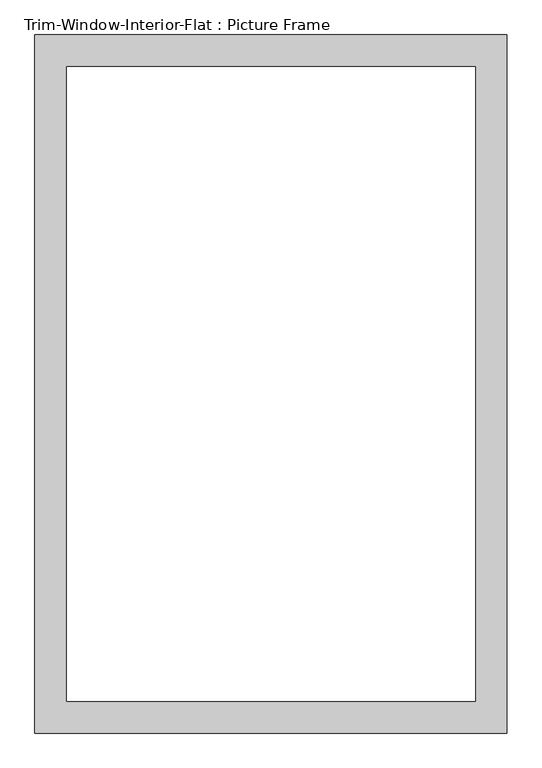
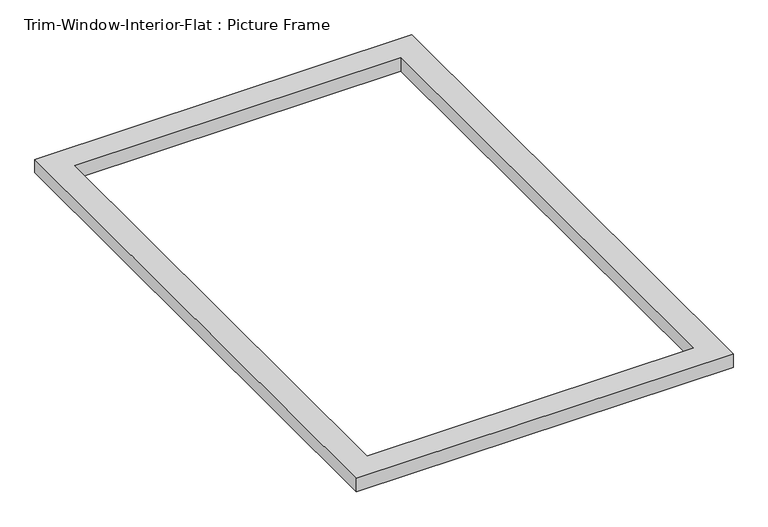
"""IFC4 building model written with IfcOpenShell, lengths in millimetres: proxy geometry, Trim-Window-Interior-Flat : Picture Frame."""

from ifc_helpers import new_model, si_unit, origin, origin_with_axes, place, context, project, spatial, polyline, outline, extrude, source, transform, mapped, element, save


def trim_window_interior_flat_picture_frame_50b64344(model_context):
    return source(origin(), model_context, "Body", "SweptSolid", [
        extrude(outline(polyline([(425.45, -44.45), (-425.45, -44.45), (-425.45, 1212.85), (425.45, 1212.85), (425.45, -44.45)]), holes=[polyline([(368.3, 12.7), (368.3, 1155.7), (-368.3, 1155.7), (-368.3, 12.7), (368.3, 12.7)])]), origin_with_axes(), (0.0, 0.0, 1.0), 31.75),
    ])


if __name__ == "__main__":
    model = new_model("IFC4")
    model_context = context("Model", 3, world=origin())
    ifc_project = project(units=[si_unit("LENGTHUNIT", "METRE", prefix="MILLI")], contexts=[model_context])
    site = spatial("IfcSite", under=ifc_project)
    building = spatial("IfcBuilding", under=site)
    placement = place(None, origin())
    trim_window_interior_flat_picture_frame_shape = trim_window_interior_flat_picture_frame_50b64344(model_context)
    element("IfcBuildingElementProxy", 1, Name="Trim-Window-Interior-Flat : Picture Frame", ObjectType="Trim-Window-Interior-Flat : Picture Frame", at=placement, inside=building, context=model_context, shape_type="MappedRepresentation", body=[
        mapped(trim_window_interior_flat_picture_frame_shape, transform((0.0, 0.0, 0.0), x_axis=(1.0, 0.0, 0.0), y_axis=(0.0, 1.0, 0.0), z_axis=(0.0, 0.0, 1.0))),
    ])
    save(model, "model.ifc")

# Revit data of these elements
# Type "Trim-Window-Interior-Flat : Picture Frame"
#   Trim Thickness_Picture Frame = 0' - 1 1/4"
#   Trim Width = 0' - 2 1/4"
#   Trim Thickness_with Sill = 0' - 0 3/4"
#   Sill Thickness = 0' - 1 1/4"
#   Opening Width [instance default] = 2' - 0"
#   Opening Height [instance default] = 3' - 0"
#   Default Elevation = 4' - 0"
#   Sill = no
#   Picture Frame = yes
#   Trim Material [instance default] = none
# Element 1 (IfcBuildingElementProxy, "Trim-Window-Interior-Flat : Picture Frame")
#   Opening Width = 2' - 6"
#   Opening Height = 3' - 10"
#   Trim Material = Wood - Stained
#   Materials on its faces: "Wood - Stained"
# Materials
#   "Wood - Stained": class "Wood", colour RGB 224 178 126, transparency 0, Cost = 0
